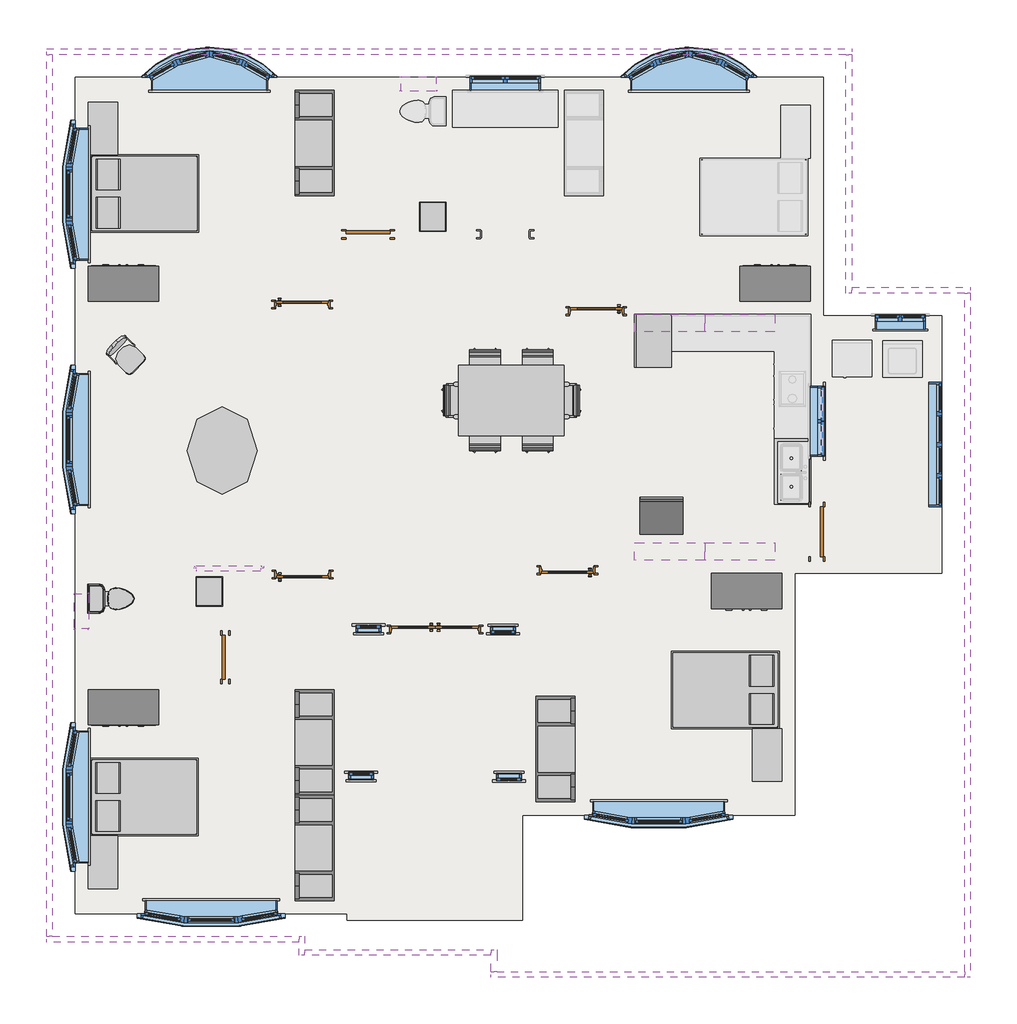
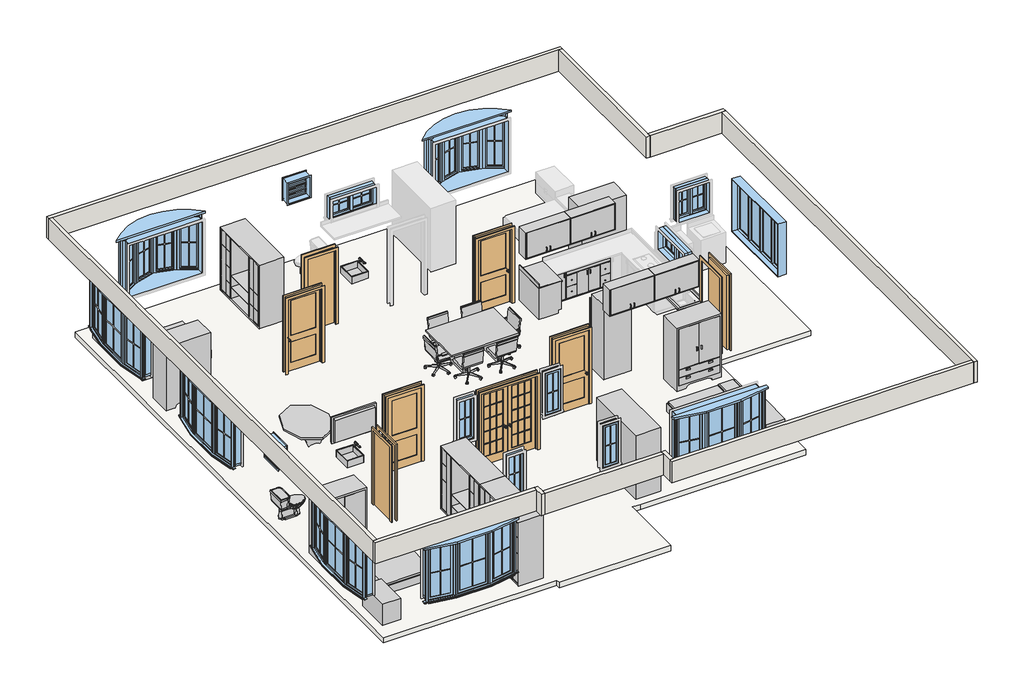
# One storey, part 1 of 2: 32 furniture elements, 17 windows, 10 walls, 8 doors, 3 flow terminals, 1 proxy, 1 slab.
"""IFC4 building model written with IfcOpenShell, lengths in millimetres."""

from ifc_helpers import new_model, si_unit, frame, origin, place, context, project, spatial, polyline, outline, extrude, faceted_brep, transform, mapped, element, save
from components import proxy_76352e5b, door_fac3bb52, door_d4071c8b, door_049a69ed, door_78caadf7, door_de72ddbf, flow_terminal_cce4e9d2, toilet_domestic_3d_toilet_domestic_3d_ba6479b0, toilet_domestic_3d_toilet_domestic_3d_30431060, furniture_b04c6994, furniture_ff3c2f57, furniture_b58f7881, furniture_6b884072, chair_task_chair_task_b7f3823b, chair_task_arms_chair_task_arms_fa5a08ef, furniture_4e2f607e, furniture_5f80dcf3, furniture_88072bd9, furniture_eb3a3c23, furniture_0bcc43ae, furniture_c105135d, furniture_5e39d705, furniture_ea954fa4, furniture_82e269c4, window_133af304, window_4630e4ac, window_bf21e6cb, window_ab94cc4f, window_791baf9d, window_a42194c0, window_f2d8fef0

model = new_model("IFC4")

# Units and contexts
model_context = context("Model", 3, world=origin())
ifc_project = project(units=[si_unit("LENGTHUNIT", "METRE", prefix="MILLI")], contexts=[model_context])

# Site, building, storey
site = spatial("IfcSite", under=ifc_project)
building = spatial("IfcBuilding", under=site)
storey = spatial("IfcBuildingStorey", under=building, Elevation=914.4)

# Proxy
placement = place(None, origin())
proxy_shape = proxy_76352e5b(model_context)
element("IfcBuildingElementProxy", 1, Name="Refrigerator-Built-in : 30\" x 24\" LH", ObjectType="Refrigerator-Built-in : 30\" x 24\" LH", at=placement, inside=storey, context=model_context, shape_type="MappedRepresentation", body=[
    mapped(proxy_shape, transform((-9990.4494093, 7653.8997772, 914.4), x_axis=(1.0, 0.0, 0.0), y_axis=(0.0, 1.0, 0.0), z_axis=(0.0, 0.0, 1.0))),
])

# Doors
door_shape = door_fac3bb52(model_context)
element("IfcDoor", 2, ObjectType="Door-Interior-Double-Full Glass-Wood : 60\" x 84\"", at=placement, inside=storey, context=model_context, shape_type="MappedRepresentation", body=[
    mapped(door_shape, transform((-13921.0994093, 5718.3487487, 914.4), x_axis=(1.0, 0.0, 0.0), y_axis=(0.0, 1.0, 0.0), z_axis=(0.0, 0.0, 1.0))),
])
door_2_shape = door_d4071c8b(model_context)
element("IfcDoor", 3, ObjectType="Door-Interior-Single-2_Panel-Wood : 36\" x 84\"", at=placement, inside=storey, context=model_context, shape_type="MappedRepresentation", body=[
    mapped(door_2_shape, transform((-16226.1494093, 11357.1487487, 914.4), x_axis=(1.0, 0.0, 0.0), y_axis=(0.0, 1.0, 0.0), z_axis=(0.0, 0.0, 1.0))),
])
element("IfcDoor", 4, ObjectType="Door-Interior-Single-2_Panel-Wood : 36\" x 84\"", at=placement, inside=storey, context=model_context, shape_type="MappedRepresentation", body=[
    mapped(door_2_shape, transform((-11622.3994093, 6740.6987487, 914.4), x_axis=(-1.0, 0.0, 0.0), y_axis=(0.0, -1.0, 0.0), z_axis=(0.0, 0.0, 1.0))),
])
door_3_shape = door_049a69ed(model_context)
element("IfcDoor", 5, ObjectType="Door-Interior-Single-2_Panel-Wood : 36\" x 84\"", at=placement, inside=storey, context=model_context, shape_type="MappedRepresentation", body=[
    mapped(door_3_shape, transform((-11120.7494093, 11242.8487487, 914.4), x_axis=(-1.0, 0.0, 0.0), y_axis=(0.0, -1.0, 0.0), z_axis=(0.0, 0.0, 1.0))),
])
element("IfcDoor", 6, ObjectType="Door-Interior-Single-2_Panel-Wood : 36\" x 84\"", at=placement, inside=storey, context=model_context, shape_type="MappedRepresentation", body=[
    mapped(door_3_shape, transform((-16219.7994093, 6664.4987487, 914.4), x_axis=(1.0, 0.0, 0.0), y_axis=(0.0, 1.0, 0.0), z_axis=(0.0, 0.0, 1.0))),
])
door_4_shape = door_78caadf7(model_context)
element("IfcDoor", 7, ObjectType="Single-Flush : 30\" x 84\"", at=placement, inside=storey, context=model_context, shape_type="MappedRepresentation", body=[
    mapped(door_4_shape, transform((-15083.1494093, 12573.1737487, 914.4), x_axis=(-1.0, 0.0, 0.0), y_axis=(0.0, -1.0, 0.0), z_axis=(0.0, 0.0, 1.0))),
])
element("IfcDoor", 8, ObjectType="Single-Flush : 30\" x 84\"", at=placement, inside=storey, context=model_context, shape_type="MappedRepresentation", body=[
    mapped(door_4_shape, transform((-17559.6494093, 5232.5737487, 914.4), x_axis=(0.0, -1.0, 0.0), y_axis=(1.0, 0.0, 0.0), z_axis=(0.0, 0.0, 1.0))),
])
door_5_shape = door_de72ddbf(model_context)
element("IfcDoor", 9, ObjectType="Single-Flush : 34\" x 84\"", at=placement, inside=storey, context=model_context, shape_type="MappedRepresentation", body=[
    mapped(door_5_shape, transform((-7291.6994093, 7410.6237487, 914.4), x_axis=(0.0, -1.0, 0.0), y_axis=(1.0, 0.0, 0.0), z_axis=(0.0, 0.0, 1.0))),
])

# Flow terminals
flow_terminal_shape = flow_terminal_cce4e9d2(model_context)
element("IfcFlowTerminal", 10, ObjectType="Sink - Work : 20\"x18\"", at=placement, inside=storey, context=model_context, shape_type="MappedRepresentation", body=[
    mapped(flow_terminal_shape, transform((-13730.5994093, 12877.9737487, 1828.8), x_axis=(0.0, -1.0, 0.0), y_axis=(1.0, 0.0, 0.0), z_axis=(0.0, 0.0, 1.0))),
])
element("IfcFlowTerminal", 11, ObjectType="Sink - Work : 20\"x18\"", at=placement, inside=storey, context=model_context, shape_type="MappedRepresentation", body=[
    mapped(flow_terminal_shape, transform((-17610.4494093, 6375.5737487, 1828.8), x_axis=(0.0, -1.0, 0.0), y_axis=(1.0, 0.0, 0.0), z_axis=(0.0, 0.0, 1.0))),
])
toilet_domestic_3d_toilet_domestic_3d_shape = toilet_domestic_3d_toilet_domestic_3d_ba6479b0(model_context)
toilet_domestic_3d_toilet_domestic_3d_2_shape = toilet_domestic_3d_toilet_domestic_3d_30431060(model_context)
element("IfcFlowTerminal", 12, ObjectType="Toilet-Domestic-3D : Toilet-Domestic-3D", at=placement, inside=storey, context=model_context, shape_type="MappedRepresentation", body=[
    mapped(toilet_domestic_3d_toilet_domestic_3d_shape, transform((-19451.3454366, 6248.5737487, 914.4), x_axis=(0.0, 1.0, 0.0), y_axis=(-1.0, 0.0, 0.0), z_axis=(0.0, 0.0, 1.0))),
    mapped(toilet_domestic_3d_toilet_domestic_3d_2_shape, transform((-19451.3454366, 6248.5737487, 914.4), x_axis=(0.0, 1.0, 0.0), y_axis=(-1.0, 0.0, 0.0), z_axis=(0.0, 0.0, 1.0))),
])

# Furniture
furniture_shape = furniture_b04c6994(model_context)
element("IfcFurniture", 13, ObjectType="48\" 2", at=placement, inside=storey, context=model_context, shape_type="MappedRepresentation", body=[
    mapped(furniture_shape, transform((-9020.8443693, 11182.5237487, 914.4), x_axis=(1.0, 0.0, 0.0), y_axis=(0.0, 1.0, 0.0), z_axis=(0.0, 0.0, 1.0))),
])
furniture_2_shape = furniture_ff3c2f57(model_context)
element("IfcFurniture", 14, ObjectType="Base Cabinet-Corner Unit-Square : 36\" 2", at=placement, inside=storey, context=model_context, shape_type="MappedRepresentation", body=[
    mapped(furniture_2_shape, transform((-10453.9994093, 10655.7860438, 914.4), x_axis=(0.0, 1.0, 0.0), y_axis=(-1.0, 0.0, 0.0), z_axis=(0.0, 0.0, 1.0))),
])
furniture_3_shape = furniture_b58f7881(model_context)
element("IfcFurniture", 15, ObjectType="Bed-Box : Double 53\" x 74\"", at=placement, inside=storey, context=model_context, shape_type="MappedRepresentation", body=[
    mapped(furniture_3_shape, transform((-19197.4289175, 12938.8712897, 914.4), x_axis=(0.0, 1.0, 0.0), y_axis=(-1.0, 0.0, 0.0), z_axis=(0.0, 0.0, 1.0))),
])
element("IfcFurniture", 16, ObjectType="Bed-Box : Double 53\" x 74\"", at=placement, inside=storey, context=model_context, shape_type="MappedRepresentation", body=[
    mapped(furniture_3_shape, transform((-19203.7789175, 2467.7212897, 914.4), x_axis=(0.0, 1.0, 0.0), y_axis=(-1.0, 0.0, 0.0), z_axis=(0.0, 0.0, 1.0))),
])
element("IfcFurniture", 17, ObjectType="Bed-Box : Double 53\" x 74\"", at=placement, inside=storey, context=model_context, shape_type="MappedRepresentation", body=[
    mapped(furniture_3_shape, transform((-8644.7699011, 5006.5762077, 914.4), x_axis=(0.0, -1.0, 0.0), y_axis=(1.0, 0.0, 0.0), z_axis=(0.0, 0.0, 1.0))),
])
furniture_4_shape = furniture_6b884072(model_context)
element("IfcFurniture", 18, ObjectType="Cabinet File-Lateral 2 Drawer : 36\" x 20\" x 24\"", at=placement, inside=storey, context=model_context, shape_type="MappedRepresentation", body=[
    mapped(furniture_4_shape, transform((-20621.2177854, 14588.3462626, 914.4), x_axis=(0.0, 1.0, 0.0), y_axis=(-1.0, 0.0, 0.0), z_axis=(0.0, 0.0, 1.0))),
])
element("IfcFurniture", 19, ObjectType="Cabinet File-Lateral 2 Drawer : 36\" x 20\" x 24\"", at=placement, inside=storey, context=model_context, shape_type="MappedRepresentation", body=[
    mapped(furniture_4_shape, transform((-20621.2177854, 1856.5962626, 914.4), x_axis=(0.0, 1.0, 0.0), y_axis=(-1.0, 0.0, 0.0), z_axis=(0.0, 0.0, 1.0))),
])
element("IfcFurniture", 20, ObjectType="Cabinet File-Lateral 2 Drawer : 36\" x 20\" x 24\"", at=placement, inside=storey, context=model_context, shape_type="MappedRepresentation", body=[
    mapped(furniture_4_shape, transform((-7220.9810332, 3357.1012348, 914.4), x_axis=(0.0, -1.0, 0.0), y_axis=(1.0, 0.0, 0.0), z_axis=(0.0, 0.0, 1.0))),
])
chair_task_chair_task_shape = chair_task_chair_task_b7f3823b(model_context)
element("IfcFurniture", 21, ObjectType="Chair-Task : Chair-Task", at=placement, inside=storey, context=model_context, shape_type="MappedRepresentation", body=[
    mapped(chair_task_chair_task_shape, transform((-11995.7585896, 10318.8196503, 914.4), x_axis=(-1.0, 0.0, 0.0), y_axis=(0.0, -1.0, 0.0), z_axis=(0.0, 0.0, 1.0))),
])
element("IfcFurniture", 22, ObjectType="Chair-Task : Chair-Task", at=placement, inside=storey, context=model_context, shape_type="MappedRepresentation", body=[
    mapped(chair_task_chair_task_shape, transform((-12277.740229, 9061.7278471, 914.4), x_axis=(1.0, 0.0, 0.0), y_axis=(0.0, 1.0, 0.0), z_axis=(0.0, 0.0, 1.0))),
])
element("IfcFurniture", 23, ObjectType="Chair-Task : Chair-Task", at=placement, inside=storey, context=model_context, shape_type="MappedRepresentation", body=[
    mapped(chair_task_chair_task_shape, transform((-12910.1585896, 10318.8196503, 914.4), x_axis=(-1.0, 0.0, 0.0), y_axis=(0.0, -1.0, 0.0), z_axis=(0.0, 0.0, 1.0))),
])
element("IfcFurniture", 24, ObjectType="Chair-Task : Chair-Task", at=placement, inside=storey, context=model_context, shape_type="MappedRepresentation", body=[
    mapped(chair_task_chair_task_shape, transform((-13192.140229, 9061.7278471, 914.4), x_axis=(1.0, 0.0, 0.0), y_axis=(0.0, 1.0, 0.0), z_axis=(0.0, 0.0, 1.0))),
])
chair_task_arms_chair_task_arms_shape = chair_task_arms_chair_task_arms_fa5a08ef(model_context)
element("IfcFurniture", 25, ObjectType="Chair-Task Arms : Chair-Task Arms", at=placement, inside=storey, context=model_context, shape_type="MappedRepresentation", body=[
    mapped(chair_task_arms_chair_task_arms_shape, transform((-13527.2953109, 9831.2645684, 914.4), x_axis=(0.0, -1.0, 0.0), y_axis=(1.0, 0.0, 0.0), z_axis=(0.0, 0.0, 1.0))),
])
element("IfcFurniture", 26, ObjectType="Chair-Task Arms : Chair-Task Arms", at=placement, inside=storey, context=model_context, shape_type="MappedRepresentation", body=[
    mapped(chair_task_arms_chair_task_arms_shape, transform((-11660.6035077, 9549.282929, 914.4), x_axis=(0.0, 1.0, 0.0), y_axis=(-1.0, 0.0, 0.0), z_axis=(0.0, 0.0, 1.0))),
])
furniture_5_shape = furniture_4e2f607e(model_context)
element("IfcFurniture", 27, ObjectType="Counter Top : 24\" Depth", at=placement, inside=storey, context=model_context, shape_type="MappedRepresentation", body=[
    mapped(furniture_5_shape, transform((-10453.9994093, 11468.5860438, 914.4), x_axis=(0.0, 1.0, 0.0), y_axis=(-1.0, 0.0, 0.0), z_axis=(0.0, 0.0, 1.0))),
])
furniture_6_shape = furniture_5f80dcf3(model_context)
element("IfcFurniture", 28, ObjectType="Counter Top w Sink : 24\" Depth", at=placement, inside=storey, context=model_context, shape_type="MappedRepresentation", body=[
    mapped(furniture_6_shape, transform((-7393.2994093, 7823.0614536, 914.4), x_axis=(0.0, -1.0, 0.0), y_axis=(1.0, 0.0, 0.0), z_axis=(0.0, 0.0, 1.0))),
])
furniture_7_shape = furniture_88072bd9(model_context)
element("IfcFurniture", 29, ObjectType="Entertainment Center.0001 : 72\" x 72\" x 24\"", at=placement, inside=storey, context=model_context, shape_type="MappedRepresentation", body=[
    mapped(furniture_7_shape, transform((-15572.0994093, 14154.3237487, 914.4), x_axis=(0.0, -1.0, 0.0), y_axis=(1.0, 0.0, 0.0), z_axis=(0.0, 0.0, 1.0))),
])
element("IfcFurniture", 30, ObjectType="Entertainment Center.0001 : 72\" x 72\" x 24\"", at=placement, inside=storey, context=model_context, shape_type="MappedRepresentation", body=[
    mapped(furniture_7_shape, transform((-12270.0994093, 3638.7237487, 914.4), x_axis=(0.0, 1.0, 0.0), y_axis=(-1.0, 0.0, 0.0), z_axis=(0.0, 0.0, 1.0))),
])
element("IfcFurniture", 31, ObjectType="Entertainment Center.0001 : 72\" x 72\" x 24\"", at=placement, inside=storey, context=model_context, shape_type="MappedRepresentation", body=[
    mapped(furniture_7_shape, transform((-15572.0994093, 1924.2237487, 914.4), x_axis=(0.0, -1.0, 0.0), y_axis=(1.0, 0.0, 0.0), z_axis=(0.0, 0.0, 1.0))),
])
element("IfcFurniture", 32, ObjectType="Entertainment Center.0001 : 72\" x 72\" x 24\"", at=placement, inside=storey, context=model_context, shape_type="MappedRepresentation", body=[
    mapped(furniture_7_shape, transform((-15572.0994093, 3753.0237487, 914.4), x_axis=(0.0, -1.0, 0.0), y_axis=(1.0, 0.0, 0.0), z_axis=(0.0, 0.0, 1.0))),
])
furniture_8_shape = furniture_eb3a3c23(model_context)
element("IfcFurniture", 33, ObjectType="Seating-Auditorium : 18\" x 24\" x 30\"", at=placement, inside=storey, context=model_context, shape_type="MappedRepresentation", body=[
    mapped(furniture_8_shape, transform((-19310.9207256, 10729.9667219, 914.4), x_axis=(-0.7071067811865499, -0.7071067811865454, 0.0), y_axis=(0.7071067811865454, -0.7071067811865499, 0.0), z_axis=(0.0, 0.0, 1.0))),
])
furniture_9_shape = furniture_0bcc43ae(model_context)
element("IfcFurniture", 34, ObjectType="Table-Conference2 w Chairs : 48\" x 144\" 2", at=placement, inside=storey, context=model_context, shape_type="MappedRepresentation", body=[
    mapped(furniture_9_shape, transform((-12593.9494093, 9690.2737487, 914.4), x_axis=(1.0, 0.0, 0.0), y_axis=(0.0, 1.0, 0.0), z_axis=(0.0, 0.0, 1.0))),
])
furniture_10_shape = furniture_c105135d(model_context)
element("IfcFurniture", 35, ObjectType="Table-Ellipse : 60\" x 48\" 2", at=placement, inside=storey, context=model_context, shape_type="MappedRepresentation", body=[
    mapped(furniture_10_shape, transform((-17616.7994093, 8820.3237487, 914.4), x_axis=(0.0, 1.0, 0.0), y_axis=(-1.0, 0.0, 0.0), z_axis=(0.0, 0.0, 1.0))),
])
furniture_11_shape = furniture_5e39d705(model_context)
element("IfcFurniture", 36, ObjectType="Television-Plasma : 50\" 2", at=placement, inside=storey, context=model_context, shape_type="MappedRepresentation", body=[
    mapped(furniture_11_shape, transform((-17445.3494093, 6724.8237487, 2133.6), x_axis=(-1.0, 0.0, 0.0), y_axis=(0.0, -1.0, 0.0), z_axis=(0.0, 0.0, 1.0))),
])
furniture_12_shape = furniture_ea954fa4(model_context)
element("IfcFurniture", 37, ObjectType="Upper Cabinet-Pass-Thru : 48\" x 30\" x 12\"", at=placement, inside=storey, context=model_context, shape_type="MappedRepresentation", body=[
    mapped(furniture_12_shape, transform((-9825.6617044, 6915.3237487, 1676.4), x_axis=(-1.0, 0.0, 0.0), y_axis=(0.0, -1.0, 0.0), z_axis=(0.0, 0.0, 1.0))),
])
element("IfcFurniture", 38, ObjectType="Upper Cabinet-Pass-Thru : 48\" x 30\" x 12\"", at=placement, inside=storey, context=model_context, shape_type="MappedRepresentation", body=[
    mapped(furniture_12_shape, transform((-8606.4617044, 6915.3237487, 1676.4), x_axis=(-1.0, 0.0, 0.0), y_axis=(0.0, -1.0, 0.0), z_axis=(0.0, 0.0, 1.0))),
])
element("IfcFurniture", 39, ObjectType="Upper Cabinet-Pass-Thru : 48\" x 30\" x 12\"", at=placement, inside=storey, context=model_context, shape_type="MappedRepresentation", body=[
    mapped(furniture_12_shape, transform((-9863.1371142, 11182.5237487, 914.4), x_axis=(1.0, 0.0, 0.0), y_axis=(0.0, 1.0, 0.0), z_axis=(0.0, 0.0, 1.0))),
])
element("IfcFurniture", 40, ObjectType="Upper Cabinet-Pass-Thru : 48\" x 30\" x 12\"", at=placement, inside=storey, context=model_context, shape_type="MappedRepresentation", body=[
    mapped(furniture_12_shape, transform((-8643.9371142, 11182.5237487, 914.4), x_axis=(1.0, 0.0, 0.0), y_axis=(0.0, 1.0, 0.0), z_axis=(0.0, 0.0, 1.0))),
])
furniture_13_shape = furniture_82e269c4(model_context)
element("IfcFurniture", 41, ObjectType="Wardrobe : 48\" x 72\" x 24\"", at=placement, inside=storey, context=model_context, shape_type="MappedRepresentation", body=[
    mapped(furniture_13_shape, transform((-8241.7061495, 6965.6625583, 914.4), x_axis=(1.0, 0.0, 0.0), y_axis=(0.0, 1.0, 0.0), z_axis=(0.0, 0.0, 1.0))),
])
element("IfcFurniture", 42, ObjectType="Wardrobe : 48\" x 72\" x 24\"", at=placement, inside=storey, context=model_context, shape_type="MappedRepresentation", body=[
    mapped(furniture_13_shape, transform((-19062.1061495, 4946.3625583, 914.4), x_axis=(1.0, 0.0, 0.0), y_axis=(0.0, 1.0, 0.0), z_axis=(0.0, 0.0, 1.0))),
])
element("IfcFurniture", 43, ObjectType="Wardrobe : 48\" x 72\" x 24\"", at=placement, inside=storey, context=model_context, shape_type="MappedRepresentation", body=[
    mapped(furniture_13_shape, transform((-19600.4926691, 11132.1849391, 914.4), x_axis=(-1.0, 0.0, 0.0), y_axis=(0.0, -1.0, 0.0), z_axis=(0.0, 0.0, 1.0))),
])
element("IfcFurniture", 44, ObjectType="Wardrobe : 48\" x 72\" x 24\"", at=placement, inside=storey, context=model_context, shape_type="MappedRepresentation", body=[
    mapped(furniture_13_shape, transform((-8284.7926691, 11132.1849391, 914.4), x_axis=(-1.0, 0.0, 0.0), y_axis=(0.0, -1.0, 0.0), z_axis=(0.0, 0.0, 1.0))),
])

# Slab
element("IfcSlab", 45, ObjectType="Generic - 6\"", at=placement, inside=storey, context=model_context, shape_type="SweptSolid", body=[
    extrude(outline(polyline([(-7177.3994093, 15297.3237487), (-7177.3994093, 11157.1237487), (-5119.9994093, 11157.1237487), (-5119.9994093, 6686.7237487), (-7672.6994093, 6686.7237487), (-7672.6994093, 2495.7237487), (-12168.4994093, 2495.7237487), (-12397.0994093, 2495.7237487), (-12397.0994093, 666.9237487), (-15445.0994093, 666.9237487), (-15445.0994093, 781.2237487), (-20169.4994093, 781.2237487), (-20169.4994093, 15297.3237487), (-7177.3994093, 15297.3237487)])), frame((0.0, 0.0, 762.0), z_axis=(0.0, 0.0, 1.0), x_axis=(1.0, 0.0, 0.0)), (0.0, 0.0, 1.0), 152.4),
])

# Walls
element("IfcWall", 46, at=placement, inside=storey, context=model_context, shape_type="Brep", body=[
    faceted_brep([(-20664.7994093, 15691.0237487, 3505.2), (-20563.1994093, 15691.0237487, 3505.2), (-6783.6994093, 15691.0237487, 3505.2), (-6682.0994093, 15691.0237487, 3505.2), (-6682.0994093, 15691.0237487, 4114.8), (-6783.6994093, 15691.0237487, 4114.8), (-20563.1994093, 15691.0237487, 4114.8), (-20664.7994093, 15691.0237487, 4114.8), (-20664.7994093, 15792.6237487, 3505.2), (-20664.7994093, 15792.6237487, 4114.8), (-6682.0994093, 15792.6237487, 4114.8), (-6682.0994093, 15792.6237487, 3505.2)], [[[0, 1, 2, 3, 4, 5, 6, 7]], [[8, 9, 10, 11]], [[3, 2, 1, 0, 8, 11]], [[7, 6, 5, 4, 10, 9]], [[4, 3, 11, 10]], [[0, 7, 9, 8]]]),
])
element("IfcWall", 47, at=placement, inside=storey, context=model_context, shape_type="Brep", body=[
    faceted_brep([(-6783.6994093, 15691.0237487, 3505.2), (-6783.6994093, 11550.8237487, 3505.2), (-6783.6994093, 11550.8237487, 4114.8), (-6783.6994093, 15691.0237487, 4114.8), (-6682.0994093, 15691.0237487, 3505.2), (-6682.0994093, 15691.0237487, 4114.8), (-6682.0994093, 11652.4237487, 4114.8), (-6682.0994093, 11550.8237487, 4114.8), (-6682.0994093, 11550.8237487, 3505.2), (-6682.0994093, 11652.4237487, 3505.2)], [[[0, 1, 2, 3]], [[4, 5, 6, 7, 8, 9]], [[1, 0, 4, 9, 8]], [[3, 2, 7, 6, 5]], [[0, 3, 5, 4]], [[2, 1, 8, 7]]]),
])
element("IfcWall", 48, at=placement, inside=storey, context=model_context, shape_type="Brep", body=[
    faceted_brep([(-6682.0994093, 11550.8237487, 3505.2), (-4726.2994093, 11550.8237487, 3505.2), (-4624.6994093, 11550.8237487, 3505.2), (-4624.6994093, 11550.8237487, 4114.8), (-4726.2994093, 11550.8237487, 4114.8), (-6682.0994093, 11550.8237487, 4114.8), (-6682.0994093, 11652.4237487, 3505.2), (-6682.0994093, 11652.4237487, 4114.8), (-4624.6994093, 11652.4237487, 4114.8), (-4624.6994093, 11652.4237487, 3505.2)], [[[0, 1, 2, 3, 4, 5]], [[6, 7, 8, 9]], [[2, 1, 0, 6, 9]], [[5, 4, 3, 8, 7]], [[0, 5, 7, 6]], [[3, 2, 9, 8]]]),
])
element("IfcWall", 49, at=placement, inside=storey, context=model_context, shape_type="Brep", body=[
    faceted_brep([(-4726.2994093, 11550.8237487, 3505.2), (-4726.2994093, -222.0762513, 3505.2), (-4726.2994093, -323.6762513, 3505.2), (-4726.2994093, -323.6762513, 4114.8), (-4726.2994093, -222.0762513, 4114.8), (-4726.2994093, 11550.8237487, 4114.8), (-4624.6994093, 11550.8237487, 3505.2), (-4624.6994093, 11550.8237487, 4114.8), (-4624.6994093, -323.6762513, 4114.8), (-4624.6994093, -323.6762513, 3505.2)], [[[0, 1, 2, 3, 4, 5]], [[6, 7, 8, 9]], [[2, 1, 0, 6, 9]], [[5, 4, 3, 8, 7]], [[0, 5, 7, 6]], [[3, 2, 9, 8]]]),
])
element("IfcWall", 50, at=placement, inside=storey, context=model_context, shape_type="Brep", body=[
    faceted_brep([(-4726.2994093, -222.0762513, 3505.2), (-12847.9494093, -222.0762513, 3505.2), (-12949.5494093, -222.0762513, 3505.2), (-12949.5494093, -222.0762513, 4114.8), (-12847.9494093, -222.0762513, 4114.8), (-4726.2994093, -222.0762513, 4114.8), (-4726.2994093, -323.6762513, 3505.2), (-4726.2994093, -323.6762513, 4114.8), (-12949.5494093, -323.6762513, 4114.8), (-12949.5494093, -323.6762513, 3505.2)], [[[0, 1, 2, 3, 4, 5]], [[6, 7, 8, 9]], [[2, 1, 0, 6, 9]], [[5, 4, 3, 8, 7]], [[0, 5, 7, 6]], [[3, 2, 9, 8]]]),
])
element("IfcWall", 51, at=placement, inside=storey, context=model_context, shape_type="Brep", body=[
    faceted_brep([(-12847.9494093, -222.0762513, 3505.2), (-12847.9494093, 158.9237487, 3505.2), (-12847.9494093, 158.9237487, 4114.8), (-12847.9494093, -222.0762513, 4114.8), (-12949.5494093, -222.0762513, 3505.2), (-12949.5494093, -222.0762513, 4114.8), (-12949.5494093, 57.3237487, 4114.8), (-12949.5494093, 158.9237487, 4114.8), (-12949.5494093, 158.9237487, 3505.2), (-12949.5494093, 57.3237487, 3505.2)], [[[0, 1, 2, 3]], [[4, 5, 6, 7, 8, 9]], [[1, 0, 4, 9, 8]], [[3, 2, 7, 6, 5]], [[0, 3, 5, 4]], [[2, 1, 8, 7]]]),
])
element("IfcWall", 52, at=placement, inside=storey, context=model_context, shape_type="SweptSolid", body=[
    extrude(outline(polyline([(-16181.6994093, 158.9237487), (-12949.5494093, 158.9237487), (-12949.5494093, 57.3237487), (-16181.6994093, 57.3237487), (-16181.6994093, 158.9237487)])), frame((0.0, 0.0, 3505.2), z_axis=(0.0, 0.0, 1.0), x_axis=(1.0, 0.0, 0.0)), (0.0, 0.0, 1.0), 609.6),
])
element("IfcWall", 53, at=placement, inside=storey, context=model_context, shape_type="Brep", body=[
    faceted_brep([(-16181.6994093, 57.3237487, 3505.2), (-16181.6994093, 158.9237487, 3505.2), (-16181.6994093, 387.5237487, 3505.2), (-16181.6994093, 387.5237487, 4114.8), (-16181.6994093, 158.9237487, 4114.8), (-16181.6994093, 57.3237487, 4114.8), (-16283.2994093, 57.3237487, 3505.2), (-16283.2994093, 57.3237487, 4114.8), (-16283.2994093, 285.9237487, 4114.8), (-16283.2994093, 387.5237487, 4114.8), (-16283.2994093, 387.5237487, 3505.2), (-16283.2994093, 285.9237487, 3505.2)], [[[0, 1, 2, 3, 4, 5]], [[6, 7, 8, 9, 10, 11]], [[2, 1, 0, 6, 11, 10]], [[5, 4, 3, 9, 8, 7]], [[0, 5, 7, 6]], [[3, 2, 10, 9]]]),
])
element("IfcWall", 54, at=placement, inside=storey, context=model_context, shape_type="Brep", body=[
    faceted_brep([(-16283.2994093, 387.5237487, 3505.2), (-20563.1994093, 387.5237487, 3505.2), (-20664.7994093, 387.5237487, 3505.2), (-20664.7994093, 387.5237487, 4114.8), (-20563.1994093, 387.5237487, 4114.8), (-16283.2994093, 387.5237487, 4114.8), (-16283.2994093, 285.9237487, 3505.2), (-16283.2994093, 285.9237487, 4114.8), (-20664.7994093, 285.9237487, 4114.8), (-20664.7994093, 285.9237487, 3505.2)], [[[0, 1, 2, 3, 4, 5]], [[6, 7, 8, 9]], [[2, 1, 0, 6, 9]], [[5, 4, 3, 8, 7]], [[0, 5, 7, 6]], [[3, 2, 9, 8]]]),
])
element("IfcWall", 55, at=placement, inside=storey, context=model_context, shape_type="SweptSolid", body=[
    extrude(outline(polyline([(-20563.1994093, 15691.0237487), (-20563.1994093, 387.5237487), (-20664.7994093, 387.5237487), (-20664.7994093, 15691.0237487), (-20563.1994093, 15691.0237487)])), frame((0.0, 0.0, 3505.2), z_axis=(0.0, 0.0, 1.0), x_axis=(1.0, 0.0, 0.0)), (0.0, 0.0, 1.0), 609.6),
])

# Windows
window_shape = window_133af304(model_context)
element("IfcWindow", 56, ObjectType="Window-Awning-Double-Horizontal : 48\" x 24\"", at=placement, inside=storey, context=model_context, shape_type="MappedRepresentation", body=[
    mapped(window_shape, transform((-12701.8994093, 15183.0237487, 914.4), x_axis=(1.0, 0.0, 0.0), y_axis=(0.0, 1.0, 0.0), z_axis=(0.0, 0.0, 1.0))),
])
element("IfcWindow", 57, ObjectType="Window-Awning-Double-Horizontal : 48\" x 24\"", at=placement, inside=storey, context=model_context, shape_type="MappedRepresentation", body=[
    mapped(window_shape, transform((-7291.6994093, 9328.3237487, 1155.7), x_axis=(0.0, -1.0, 0.0), y_axis=(1.0, 0.0, 0.0), z_axis=(0.0, 0.0, 1.0))),
])
window_2_shape = window_4630e4ac(model_context)
element("IfcWindow", 58, ObjectType="Window-Awning-Single : 17\" x 48\"", at=placement, inside=storey, context=model_context, shape_type="MappedRepresentation", body=[
    mapped(window_2_shape, transform((-12638.3994093, 3162.4737487, 914.4), x_axis=(-1.0, 0.0, 0.0), y_axis=(0.0, -1.0, 0.0), z_axis=(0.0, 0.0, 1.0))),
])
element("IfcWindow", 59, ObjectType="Window-Awning-Single : 17\" x 48\"", at=placement, inside=storey, context=model_context, shape_type="MappedRepresentation", body=[
    mapped(window_2_shape, transform((-15203.7994093, 3162.4737487, 914.4), x_axis=(1.0, 0.0, 0.0), y_axis=(0.0, 1.0, 0.0), z_axis=(0.0, 0.0, 1.0))),
])
element("IfcWindow", 60, ObjectType="Window-Awning-Single : 17\" x 48\"", at=placement, inside=storey, context=model_context, shape_type="MappedRepresentation", body=[
    mapped(window_2_shape, transform((-15076.7994093, 5715.1737487, 914.4), x_axis=(1.0, 0.0, 0.0), y_axis=(0.0, 1.0, 0.0), z_axis=(0.0, 0.0, 1.0))),
])
element("IfcWindow", 61, ObjectType="Window-Awning-Single : 17\" x 48\"", at=placement, inside=storey, context=model_context, shape_type="MappedRepresentation", body=[
    mapped(window_2_shape, transform((-12739.9994093, 5715.1737487, 914.4), x_axis=(-1.0, 0.0, 0.0), y_axis=(0.0, -1.0, 0.0), z_axis=(0.0, 0.0, 1.0))),
])
window_3_shape = window_bf21e6cb(model_context)
element("IfcWindow", 62, ObjectType="Window-Bay-Casement-10_Degree_Angle : 90\" x 60\" x 6\"", at=placement, inside=storey, context=model_context, shape_type="MappedRepresentation", body=[
    mapped(window_3_shape, transform((-20055.1994093, 13268.4987487, 914.4), x_axis=(0.0, 1.0, 0.0), y_axis=(-1.0, 0.0, 0.0), z_axis=(0.0, 0.0, 1.0))),
])
element("IfcWindow", 63, ObjectType="Window-Bay-Casement-10_Degree_Angle : 90\" x 60\" x 6\"", at=placement, inside=storey, context=model_context, shape_type="MappedRepresentation", body=[
    mapped(window_3_shape, transform((-20055.1994093, 9010.8237487, 914.4), x_axis=(0.0, 1.0, 0.0), y_axis=(-1.0, 0.0, 0.0), z_axis=(0.0, 0.0, 1.0))),
])
element("IfcWindow", 64, ObjectType="Window-Bay-Casement-10_Degree_Angle : 90\" x 60\" x 6\"", at=placement, inside=storey, context=model_context, shape_type="MappedRepresentation", body=[
    mapped(window_3_shape, transform((-20055.1994093, 2810.0487487, 914.4), x_axis=(0.0, 1.0, 0.0), y_axis=(-1.0, 0.0, 0.0), z_axis=(0.0, 0.0, 1.0))),
])
element("IfcWindow", 65, ObjectType="Window-Bay-Casement-10_Degree_Angle : 90\" x 60\" x 6\"", at=placement, inside=storey, context=model_context, shape_type="MappedRepresentation", body=[
    mapped(window_3_shape, transform((-17807.2994093, 895.5237487, 914.4), x_axis=(-1.0, 0.0, 0.0), y_axis=(0.0, -1.0, 0.0), z_axis=(0.0, 0.0, 1.0))),
])
element("IfcWindow", 66, ObjectType="Window-Bay-Casement-10_Degree_Angle : 90\" x 60\" x 6\"", at=placement, inside=storey, context=model_context, shape_type="MappedRepresentation", body=[
    mapped(window_3_shape, transform((-10034.8994093, 2610.0237487, 914.4), x_axis=(-1.0, 0.0, 0.0), y_axis=(0.0, -1.0, 0.0), z_axis=(0.0, 0.0, 1.0))),
])
window_4_shape = window_ab94cc4f(model_context)
element("IfcWindow", 67, ObjectType="Window-Bow-Casement-15_Degree_Angle : 80\" x 60\"", at=placement, inside=storey, context=model_context, shape_type="MappedRepresentation", body=[
    mapped(window_4_shape, transform((-17835.8744093, 15183.0237487, 914.4), x_axis=(1.0, 0.0, 0.0), y_axis=(0.0, 1.0, 0.0), z_axis=(0.0, 0.0, 1.0))),
])
element("IfcWindow", 68, ObjectType="Window-Bow-Casement-15_Degree_Angle : 80\" x 60\"", at=placement, inside=storey, context=model_context, shape_type="MappedRepresentation", body=[
    mapped(window_4_shape, transform((-9511.0244093, 15183.0237487, 914.4), x_axis=(1.0, 0.0, 0.0), y_axis=(0.0, 1.0, 0.0), z_axis=(0.0, 0.0, 1.0))),
])
window_5_shape = window_791baf9d(model_context)
element("IfcWindow", 69, ObjectType="Window-Casement-Double : 34\" x 36\"", at=placement, inside=storey, context=model_context, shape_type="MappedRepresentation", body=[
    mapped(window_5_shape, transform((-5843.8994093, 11042.8237487, 914.4), x_axis=(-1.0, 0.0, 0.0), y_axis=(0.0, -1.0, 0.0), z_axis=(0.0, 0.0, 1.0))),
])
window_6_shape = window_a42194c0(model_context)
element("IfcWindow", 70, ObjectType="Window-Casement-Multi-Sash-Horizontal : 85\" x 60\"", at=placement, inside=storey, context=model_context, shape_type="MappedRepresentation", body=[
    mapped(window_6_shape, transform((-5234.2994093, 8921.9237487, 914.4), x_axis=(0.0, -1.0, 0.0), y_axis=(1.0, 0.0, 0.0), z_axis=(0.0, 0.0, 1.0))),
])
window_7_shape = window_f2d8fef0(model_context)
element("IfcWindow", 71, ObjectType="Window-Louvers : 24\" x 24\"", at=placement, inside=storey, context=model_context, shape_type="MappedRepresentation", body=[
    mapped(window_7_shape, transform((-20061.5494093, 6032.6737487, 1828.8), x_axis=(0.0, 1.0, 0.0), y_axis=(-1.0, 0.0, 0.0), z_axis=(0.0, 0.0, 1.0))),
])
element("IfcWindow", 72, ObjectType="Window-Louvers : 24\" x 24\"", at=placement, inside=storey, context=model_context, shape_type="MappedRepresentation", body=[
    mapped(window_7_shape, transform((-14206.8494093, 15189.3737487, 1828.8), x_axis=(1.0, 0.0, 0.0), y_axis=(0.0, 1.0, 0.0), z_axis=(0.0, 0.0, 1.0))),
])

save(model, "model.ifc")

# Revit data of these elements
# Type "Refrigerator-Built-in : 30\" x 24\" LH"
#   Assembly Code = "E1090400"
#   Depth = 2' - 0"
#   Handle = 0' - 0 1/4"
#   Height = 7' - 0"
#   Top Door Height = 5' - 0"
#   Width = 2' - 5 1/2"
#   Material = Metal - Paint Finish - Ivory,Glossy
#   Default Elevation = 0
# Type "Door-Interior-Double-Full Glass-Wood : 60\" x 84\""
#   Type Mark = "9"
#   Assembly Code = "C1020300"
#   Analytic Construction = "French door, wood frame with single glass"
#   Top Rail = 0' - 4 11/16"
#   Thickness = 0' - 1 3/8"
#   Thermal Resistance (R) = 1.0696 (h·ft²·°F)/BTU
#   Swing Angle [instance default] = 90.00°
#   Stiles = 0' - 4 3/4"
#   Rough Width = 5' - 2"
#   Rough Height = 7' - 1"
#   Panel Width = 2' - 6"
#   Height = 7' - 0"
#   Width = 5' - 0"
#   Heat Transfer Coefficient (U) = 0.9350 BTU/(h·ft²·°F)
#   Bottom Rail = 0' - 9 1/8"
#   Show Grill [instance default] = yes
#   Trim Material = Cherry
#   Panel Material = Cherry
#   Frame Material = Cherry
#   Door Handle Material = Aluminum
#   Visual Light Transmittance = 0
#   Solar Heat Gain Coefficient = 0
#   Wall Closure = (empty or 0)
#   Function = (empty or 0)
# Type "Door-Interior-Single-2_Panel-Wood : 36\" x 84\""
#   Type Mark = "12"
#   Assembly Code = "C1020300"
#   Analytic Construction = "Wooden"
#   Top Rail = 0' - 4 11/16"
#   Thickness = 0' - 1 3/8"
#   Thermal Resistance (R) = 2.5876 (h·ft²·°F)/BTU
#   Swing Angle [instance default] = 90.00°
#   Stiles = 0' - 4 3/4"
#   Rough Width = 3' - 2"
#   Rough Height = 7' - 1"
#   Lock Rail = 0' - 7 1/2"
#   Height = 7' - 0"
#   Width = 3' - 0"
#   Heat Transfer Coefficient (U) = 0.3865 BTU/(h·ft²·°F)
#   Bottom Rail = 0' - 9 1/8"
#   Trim Material = Cherry
#   Panel Material = Cherry
#   Frame Material = Cherry
#   Door Handle Material = Aluminum
#   Visual Light Transmittance = 0
#   Solar Heat Gain Coefficient = 0
#   Wall Closure = (empty or 0)
#   Function = (empty or 0)
# Type "Single-Flush : 30\" x 84\""
#   Type Mark = "4"
#   Construction Type Id = "MDOOR"
#   Assembly Code = "C1020"
#   Analytic Construction = "Metal"
#   Thickness = 0' - 2"
#   Heat Transfer Coefficient (U) = 0.651978 BTU/(h·ft²·°F)
#   Height = 7' - 0"
#   Trim Projection Ext = 0' - 1"
#   Trim Projection Int = 0' - 1"
#   Trim Width = 0' - 3"
#   Width = 2' - 6"
#   Define Thermal Properties by = 1
#   Define Thermal Properties by = 1
#   Door Material = Door - Panel
#   Frame Material = Door - Frame
#   Visual Light Transmittance = 0
#   Solar Heat Gain Coefficient = 0
#   Function = (empty or 0)
#   Wall Closure = (empty or 0)
# Type "Single-Flush : 34\" x 84\""
#   Type Mark = "2"
#   Construction Type Id = "MDOOR"
#   Assembly Code = "C1020"
#   Analytic Construction = "Metal"
#   Thickness = 0' - 2"
#   Heat Transfer Coefficient (U) = 0.651978 BTU/(h·ft²·°F)
#   Height = 7' - 0"
#   Trim Projection Ext = 0' - 1"
#   Trim Projection Int = 0' - 1"
#   Trim Width = 0' - 3"
#   Width = 2' - 10"
#   Define Thermal Properties by = 1
#   Define Thermal Properties by = 1
#   Door Material = Door - Panel
#   Frame Material = Door - Frame
#   Visual Light Transmittance = 0
#   Solar Heat Gain Coefficient = 0
#   Function = (empty or 0)
#   Wall Closure = (empty or 0)
# Type "Sink - Work : 20\"x18\""
#   WFU = 2
#   Sink Width = 1' - 6"
#   Sink Length = 1' - 8"
#   Sink Depth = 0' - 8"
#   Sanitary Radius = 3/4"
#   Sanitary Diameter = 1 1/2"
#   Hot Water Radius = 1/4"
#   Hot Water Diameter = 1/2"
#   HWFU = 2.25
#   Flow Pressure [instance default] = 8.00 psi
#   Faucet Height = 1' - 1 5/8"
#   Cold Water Radius = 1/4"
#   Cold Water Diameter = 1/2"
#   CWFU = 2.25
#   Sink Material = none
#   Faucet Material = none
#   Default Elevation = 0
# Type "Toilet-Domestic-3D : Toilet-Domestic-3D"
#   Assembly Code = "D2010110"
#   Toilet - Bowl/Basin Material = Porcelain, Linen
#   Toilet - Seat Material = Laminate, Linen, Matte
#   Default Elevation = 0
# Type "48\" 2"
#   Assembly Code = "C1030410"
#   Depth = 2' - 0"
#   Height = 2' - 11 1/2"
#   Toe Depth = 0' - 3"
#   Toe Height = 0' - 3 1/2"
#   Width = 4' - 0"
#   Cabinet Material = none
#   Door/Drawer Material = none
#   Handle Material = Cabinets - Handles
#   Default Elevation = 0
# Type "Base Cabinet-Corner Unit-Square : 36\" 2"
#   Assembly Code = "C1030410"
#   Depth = 2' - 0"
#   Height = 2' - 11 1/2"
#   Toe Depth = 0' - 3"
#   Toe Height = 0' - 3 1/2"
#   Width = 3' - 0"
#   Cabinet Material = Cabinets
#   Door/Drawer Material = Cabinets
#   Handle Material = Cabinets - Handles
#   Default Elevation = 0
# Type "Bed-Box : Double 53\" x 74\""
#   Assembly Code = "E2020200"
#   Length = 6' - 2"
#   Width = 4' - 5"
#   Frame Material = Birch
#   Mattress Material = Linen, White
#   Default Elevation = 0
# Type "Cabinet File-Lateral 2 Drawer : 36\" x 20\" x 24\""
#   Assembly Code = "E2020200"
#   Depth = 1' - 8"
#   Height = 2' - 0"
#   Width = 3' - 0"
#   Material = Metal - Steel
#   Default Elevation = 0
# Type "Chair-Task : Chair-Task"
#   Assembly Code = "E2020200"
#   Base Material = Plastic - Black
#   Caster Material = Plastic - Black
#   Seat/Back Material = Textile - Slate Blue
#   Default Elevation = 0
# Type "Chair-Task Arms : Chair-Task Arms"
#   Assembly Code = "E2020200"
#   Base Material = Plastic - Black
#   Caster Material = Plastic - Black
#   Seat/Back Material = Textile - Slate Blue
#   Default Elevation = 0
# Type "Counter Top : 24\" Depth"
#   Assembly Code = "C1030400"
#   Counter Thickness = 0' - 1 1/2"
#   Depth = 2' - 1"
#   Height = 3' - 0"
#   Length [instance default] = 8' - 0"
#   Counter Top Material = none
#   Default Elevation = 0
# Type "Counter Top w Sink : 24\" Depth"
#   Assembly Code = "C1030400"
#   Counter Thickness = 0' - 1 1/2"
#   Depth = 2' - 1"
#   Height = 3' - 0"
#   Length [instance default] = 8' - 0"
#   Sink Location [instance default] = 2' - 0"
#   Sink Location To Wall [instance default] = 0' - 6"
#   Sink Opening Depth [instance default] = 1' - 3"
#   Sink Opening Width [instance default] = 3' - 3"
#   Counter Top Material = none
#   Default Elevation = 0
# Type "Entertainment Center.0001 : 72\" x 72\" x 24\""
#   Assembly Code = "E2020200"
#   Center Width = 2' - 8"
#   Depth = 2' - 0"
#   Height = 6' - 0"
#   Width = 6' - 0"
#   Material = none
#   Default Elevation = 0
# Type "Seating-Auditorium : 18\" x 24\" x 30\""
#   Assembly Code = "E2020200"
#   Seat Material = Linen, Beige
#   Frame Material = Steel, Paint Finish, Dark Gray, Matte
#   Default Elevation = 0
# Type "Table-Conference2 w Chairs : 48\" x 144\" 2"
#   Assembly Code = "E2020200"
#   Description = "Seating 12-14"
#   Height = 2' - 6"
#   Length = 6' - 0"
#   Width = 4' - 0"
#   Number Of Chairs One Side = 2
#   Number Of Chairs = 6
#   Material = Wood - Cherry
#   Default Elevation = 0
# Type "Table-Ellipse : 60\" x 48\" 2"
#   Assembly Code = "E2020200"
#   Half Width = 2' - 0"
#   Half Length = 2' - 6"
#   Height = 1' - 6"
#   Length = 5' - 0"
#   Width = 4' - 0"
#   Base Material = Birch
#   Top Material = Birch
#   Default Elevation = 0
# Type "Television-Plasma : 50\" 2"
#   Assembly Code = "E2020200"
#   Depth = 0' - 3 1/2"
#   Height = 2' - 6"
#   Width = 3' - 11 1/2"
#   Cabinet Material = Plastic - Gray
#   Default Elevation = 0
# Type "Upper Cabinet-Pass-Thru : 48\" x 30\" x 12\""
#   Depth = 1' - 0"
#   Height = 2' - 6"
#   Top of Cabinet = 7' - 0"
#   Width = 4' - 0"
#   Default Elevation = 0
# Type "Wardrobe : 48\" x 72\" x 24\""
#   Assembly Code = "E2020200"
#   Depth = 2' - 0"
#   Height = 6' - 0"
#   Width = 4' - 0"
#   Material = Wood - Mahogany
#   Default Elevation = 0
# Type "Generic - 6\""
#   Assembly Code = "B1010"
#   Function = 0
#   Layers, outside or top first: 0' - 6" "Concrete, Cast-in-Place gray" (function 1)
# Type
#   Assembly Code = "B2010"
#   Layers, outside or top first: 0' - 4" "Wood - Mahogany" (function 1)
# Type "Window-Awning-Double-Horizontal : 48\" x 24\""
#   Type Mark = "20"
#   Fire Rating = "0.5h"
#   Assembly Code = "B2020100"
#   Analytic Construction = "Double glazing - domestic"
#   Window Inset [instance default] = 0' - 0"
#   Wall Thickness [instance default] = 0' - 6"
#   Interior Wall Closure [instance default] = 0' - 2 1/4"
#   Half Width = 2' - 0"
#   Visual Light Transmittance = 0.81
#   Thermal Resistance (R) = 1.8146 (h·ft²·°F)/BTU
#   Solar Heat Gain Coefficient = 0.76
#   Rough Width = 4' - 0 1/2"
#   Rough Height = 2' - 0 1/2"
#   Height = 2' - 0"
#   Heat Transfer Coefficient (U) = 0.5511 BTU/(h·ft²·°F)
#   Frame Extension [instance default] = 0' - 0 1/4"
#   Exterior Wall Closure [instance default] = 0' - 1 1/4"
#   Extension Jamb [instance default] = 0' - 2 1/4"
#   Default Sill Height = 3' - 0"
#   Width = 4' - 0"
#   Muntin Visibility = yes
#   Interior Trim Visibility [instance default] = yes
#   Exterior Trim Visibility [instance default] = yes
#   Extension Jamb Visibility [instance default] = yes
#   Interior Trim Material = Wood - Stained
#   Muntin Pattern = Muntin Pattern_2x2 : Muntin Pattern_2x2
#   Interior Trim = Trim-Window-Interior-Flat : Picture Frame
#   Interior Frame Material = Wood - Stained
#   Glass Panel Material = Glass
#   Exterior Trim Material = Clad - White
#   Exterior Trim = Trim-Window-Exterior-Flat : with Sill
#   Exterior Frame Material = Clad - White
#   Wall Closure = (empty or 0)
# Type "Window-Awning-Single : 17\" x 48\""
#   Type Mark = "27"
#   Fire Rating = "0.5h"
#   Assembly Code = "B2020100"
#   Analytic Construction = "Double glazing - domestic"
#   Window Inset [instance default] = 0' - 0"
#   Wall Thickness [instance default] = 0' - 6"
#   Visual Light Transmittance = 0.81
#   Thermal Resistance (R) = 1.8146 (h·ft²·°F)/BTU
#   Solar Heat Gain Coefficient = 0.76
#   Rough Width = 1' - 5 1/2"
#   Rough Height = 4' - 0 1/2"
#   Interior Wall Closure [instance default] = 0' - 2 1/4"
#   Height = 4' - 0"
#   Heat Transfer Coefficient (U) = 0.5511 BTU/(h·ft²·°F)
#   Frame Extension [instance default] = 0' - 0 1/4"
#   Exterior Wall Closure [instance default] = 0' - 1 1/4"
#   Extension Jamb [instance default] = 0' - 2 1/4"
#   Default Sill Height = 3' - 0"
#   Width = 1' - 5"
#   Muntin Visibility = yes
#   Interior Trim Visibility [instance default] = yes
#   Exterior Trim Visibility [instance default] = yes
#   Extension Jamb Visibility [instance default] = yes
#   Muntin Pattern = Muntin Pattern_2x2 : Muntin Pattern_2x2
#   Interior Trim Material = Wood - Stained
#   Interior Trim = Trim-Window-Interior-Flat : Picture Frame
#   Interior Frame Material = Wood - Stained
#   Glass Panel Material = Glass
#   Exterior Trim Material = Clad - White
#   Exterior Trim = Trim-Window-Exterior-Flat : with Sill
#   Exterior Frame Material = Clad - White
#   Wall Closure = (empty or 0)
# Type "Window-Bay-Casement-10_Degree_Angle : 90\" x 60\" x 6\""
#   Type Mark = "18"
#   Fire Rating = "0.5h"
#   Assembly Code = "B2020100"
#   Analytic Construction = "Double glazing - domestic"
#   Width of Middle Sash = 2' - 9.07789"
#   Width = 7' - 6"
#   Visual Light Transmittance = 0.81
#   Thermal Resistance (R) = 1.8146 (h·ft²·°F)/BTU
#   Solar Heat Gain Coefficient = 0.76
#   Rough Width = 7' - 6 1/2"
#   Rough Height = 5' - 0 1/2"
#   Length 4 = 0' - 0.24059"
#   Length 3 = 0' - 0 7/64"
#   Length 2 = 3' - 1.29661"
#   Length 1 = 2' - 2.46106"
#   Wall Thickness [instance default] = 0' - 6"
#   Trim Width = 7' - 10.21872"
#   Trim Height = 5' - 0"
#   Height 1 = 5' - 2"
#   Height = 5' - 0"
#   Heat Transfer Coefficient (U) = 0.5511 BTU/(h·ft²·°F)
#   Depth = 0' - 6"
#   Default Sill Height = 2' - 0"
#   Angle 1 = 5.00°
#   Angle = 10.00°
#   Center Muntin Visibility = yes
#   Side Muntin Visibility = yes
#   Interior Trim Visibility [instance default] = yes
#   Exterior Trim Visibility [instance default] = yes
#   Center Muntin Pattern = Muntin Pattern_2x2 : Muntin Pattern_2x2
#   Side Muntin Pattern = Muntin Pattern_2x2 : Muntin Pattern_2x2
#   Interior Trim Material = Wood - Stained
#   Exterior Trim Material = Clad - White
#   Exterior Trim = element 390327
#   Interior Trim = Trim-Window-Interior-Flat : Picture Frame
#   Interior Frame Material = Wood - Stained
#   Glass Panel Material = Glass
#   Exterior Frame Material = Clad - White
#   Wall Closure = (empty or 0)
# Type "Window-Bow-Casement-15_Degree_Angle : 80\" x 60\""
#   Type Mark = "19"
#   Fire Rating = "0.5h"
#   Assembly Code = "B2020100"
#   Analytic Construction = "Double glazing - domestic"
#   Width = 6' - 7.30579"
#   Visual Light Transmittance = 0.81
#   Thermal Resistance (R) = 1.8146 (h·ft²·°F)/BTU
#   Solar Heat Gain Coefficient = 0.76
#   Rough Width = 6' - 7.80579"
#   Rough Height = 5' - 0 1/2"
#   Length 3 = 0' - 1 239/256"
#   Height 1 = 5' - 2"
#   Height = 5' - 0"
#   Heat Transfer Coefficient (U) = 0.5511 BTU/(h·ft²·°F)
#   Depth 7 = 0' - 0 83/128"
#   Depth 6 = 0' - 1 207/256"
#   Depth 5 = 0' - 2.16481"
#   Depth 4 = 0' - 1.16481"
#   Width of Middle Sash = 3' - 5.22785"
#   Radius 2 = 5' - 4.63151"
#   Radius 1 = 5' - 3.63151"
#   Length 2 = 7' - 3.05579"
#   Length 1 = 1' - 5.10538"
#   Wall Thickness [instance default] = 0' - 6"
#   Trim Width = 6' - 11.97766"
#   Depth 3 = 0' - 5.00538"
#   Depth 2 = 0' - 6.16554"
#   Depth 1 = 0' - 11.83446"
#   Depth = 1' - 6"
#   Default Sill Height = 2' - 0"
#   Angle 2 = 15.00°
#   Angle 1 = 30.00°
#   Muntin Visibility = yes
#   Interior Trim Visibility [instance default] = yes
#   Exterior Trim Visibility [instance default] = yes
#   Interior Trim Material = Wood - Stained
#   Exterior Trim Material = Clad - White
#   Muntin Pattern = Muntin Pattern_2x2 : Muntin Pattern_2x2
#   Exterior Trim = element 398010
#   Interior Trim = Trim-Window-Interior-Flat : Picture Frame
#   Interior Frame Material = Wood - Stained
#   Glass Panel Material = Glass
#   Exterior Frame Material = Clad - White
#   Wall Closure = (empty or 0)
# Type "Window-Casement-Double : 34\" x 36\""
#   Type Mark = "14"
#   Fire Rating = "0.5h"
#   Assembly Code = "B2020100"
#   Analytic Construction = "Double glazing - domestic"
#   Frame Extension [instance default] = 0' - 0 1/4"
#   Window Inset [instance default] = 0' - 0"
#   Wall Thickness [instance default] = 0' - 6"
#   Interior Wall Closure [instance default] = 0' - 2 1/4"
#   Half Width = 1' - 5"
#   Visual Light Transmittance = 0.81
#   Thermal Resistance (R) = 1.8146 (h·ft²·°F)/BTU
#   Solar Heat Gain Coefficient = 0.76
#   Rough Width = 2' - 10 1/2"
#   Rough Height = 3' - 0 1/2"
#   Height = 3' - 0"
#   Heat Transfer Coefficient (U) = 0.5511 BTU/(h·ft²·°F)
#   Exterior Wall Closure [instance default] = 0' - 1 1/4"
#   Extension Jamb [instance default] = 0' - 2 1/4"
#   Default Sill Height = 3' - 0"
#   Width = 2' - 10"
#   Define Thermal Properties by = 0
#   Muntin Visibility = yes
#   Interior Trim Visibility [instance default] = yes
#   Exterior Trim Visibility [instance default] = yes
#   Extension Jamb Visibility [instance default] = yes
#   Interior Trim Material = Wood - Stained
#   Muntin Pattern = Muntin Pattern_2x2 : Muntin Pattern_2x2
#   Interior Trim = Trim-Window-Interior-Flat : Picture Frame
#   Interior Frame Material = Wood - Stained
#   Glass Panel Material = Glass
#   Exterior Trim Material = Clad - White
#   Exterior Trim = Trim-Window-Exterior-Flat : with Sill
#   Exterior Frame Material = Clad - White
#   Wall Closure = (empty or 0)
# Type "Window-Casement-Multi-Sash-Horizontal : 85\" x 60\""
#   Type Mark = "24"
#   Fire Rating = "0.5h"
#   Assembly Code = "B2020100"
#   Analytic Construction = "Double glazing - domestic"
#   Window Inset [instance default] = 0' - 0 5/8"
#   Wall Thickness [instance default] = 0' - 6"
#   Visual Light Transmittance = 0.81
#   Thermal Resistance (R) = 1.8146 (h·ft²·°F)/BTU
#   Solar Heat Gain Coefficient = 0.76
#   Rough Width = 7' - 1 1/2"
#   Rough Height = 5' - 0 1/2"
#   Open Window Width = 1' - 9 1/4"
#   Heat Transfer Coefficient (U) = 0.5511 BTU/(h·ft²·°F)
#   Height = 5' - 0"
#   Frame Gap 3 [instance default] = 0' - 1 83/128"
#   Frame Gap 2 [instance default] = 0' - 0 5/8"
#   Frame Gap 1 = 0' - 1 51/128"
#   Default Sill Height = 3' - 0"
#   Width = 7' - 1"
#   Frame Material = Metal - Aluminum
#   Glass Panel Material = Glass
#   Wall Closure = (empty or 0)
# Type "Window-Louvers : 24\" x 24\""
#   Type Mark = "25"
#   Construction Type Id = "GSP4R"
#   Assembly Code = "B20"
#   Analytic Construction = "1/8 in Pilkington single glazing"
#   Visual Light Transmittance = 0.9
#   Thermal Resistance (R) = 1.53941 (h·ft²·°F)/BTU
#   Solar Heat Gain Coefficient = 0.78
#   Max Height = 1' - 11.74264"
#   Height = 2' - 0"
#   Heat Transfer Coefficient (U) = 0.6496 BTU/(h·ft²·°F)
#   Blade Width [instance default] = 1' - 10 1/2"
#   Blade Vertical Thickness = 0' - 0.35355"
#   Blade Thickness = 0' - 0 1/4"
#   Blade Spacing = 0' - 1 1/2"
#   Blade Height = 0' - 1.85355"
#   Blade Depth = 0' - 3"
#   Blade Angle = 45.00°
#   Default Sill Height = 3' - 0"
#   Trim Projection_Exterior = 0' - 0 1/2"
#   Trim Projection_Interior = 0' - 0 1/2"
#   Trim Width_Exterior = 0' - 1 1/2"
#   Trim Width_Interior = 0' - 1 1/2"
#   Width = 2' - 0"
#   Max Blade Count = 12
#   Define Thermal Properties by = 1
#   Blade Count = 12
#   Frame Material = Birch
#   Louver Material = Birch
#   Trim Exterior Material = Birch
#   Trim Interior Material = Birch
#   Wall Closure = (empty or 0)
# Element 1 (IfcBuildingElementProxy, "Refrigerator-Built-in : 30\" x 24\" LH")
#   Phase Created = New Construction
#   Materials on its faces: "Metal - Paint Finish - Ivory,Glossy", "Metal - Chrome"
# Element 2 (IfcDoor, "Door-Interior-Double-Full Glass-Wood : 60\" x 84\"")
#   Swing Angle = 90.00°
#   Show Grill = yes
#   Phase Created = New Construction
#   Materials on its faces: "Cherry", "Aluminum", "Glass"
# Elements 3, 4, 5, 6 (IfcDoor, "Door-Interior-Single-2_Panel-Wood : 36\" x 84\"")
#   Swing Angle = 90.00°
#   Phase Created = New Construction
#   Materials on its faces: "Cherry", "Aluminum"
# Elements 7, 8 (IfcDoor, "Single-Flush : 30\" x 84\"")
#   Phase Created = New Construction
#   Materials on its faces: "Door - Frame", "Door - Panel"
# Element 9 (IfcDoor, "Single-Flush : 34\" x 84\"")
#   Phase Created = New Construction
#   Materials on its faces: "Door - Frame", "Door - Panel"
# Element 10 (IfcFlowTerminal, "Sink - Work : 20\"x18\"")
#   Mark = "4"
#   Flow Pressure = 8.00 psi
#   Phase Created = New Construction
# Element 11 (IfcFlowTerminal, "Sink - Work : 20\"x18\"")
#   Mark = "5"
#   Flow Pressure = 8.00 psi
#   Phase Created = New Construction
# Element 12 (IfcFlowTerminal, "Toilet-Domestic-3D : Toilet-Domestic-3D")
#   Mark = "2"
#   Phase Created = New Construction
#   Materials on its faces: "Porcelain, Linen", "Laminate, Linen, Matte"
# Element 13 (IfcFurniture, "48\" 2")
#   Phase Created = New Construction
#   Materials on its faces: "Cabinets", "Cabinets - Handles"
# Element 14 (IfcFurniture, "Base Cabinet-Corner Unit-Square : 36\" 2")
#   Phase Created = New Construction
#   Materials on its faces: "Cabinets", "Cabinets - Handles"
# Elements 15, 16, 17 (IfcFurniture, "Bed-Box : Double 53\" x 74\"")
#   Phase Created = New Construction
#   Materials on its faces: "Birch", "Linen, White"
# Elements 18, 19, 20 (IfcFurniture, "Cabinet File-Lateral 2 Drawer : 36\" x 20\" x 24\"")
#   Phase Created = New Construction
#   Materials on its faces: "Metal - Steel"
# Elements 21, 22, 23, 24 (IfcFurniture, "Chair-Task : Chair-Task")
#   Phase Created = New Construction
#   Materials on its faces: "Plastic - Black", "Textile - Slate Blue"
# Elements 25, 26 (IfcFurniture, "Chair-Task Arms : Chair-Task Arms")
#   Phase Created = New Construction
#   Materials on its faces: "Plastic - Black", "Textile - Slate Blue"
# Element 27 (IfcFurniture, "Counter Top : 24\" Depth")
#   Length = 3' - 0"
#   Phase Created = New Construction
#   Materials on its faces: "Counter Top"
# Element 28 (IfcFurniture, "Counter Top w Sink : 24\" Depth")
#   Sink Opening Width = 3' - 3"
#   Sink Opening Depth = 1' - 3"
#   Sink Location To Wall = 0' - 6"
#   Sink Location = 1' - 11"
#   Length = 3' - 8.8035"
#   Phase Created = New Construction
#   Materials on its faces: "Counter Top"
# Elements 29, 30, 31, 32 (IfcFurniture, "Entertainment Center.0001 : 72\" x 72\" x 24\"")
#   Phase Created = New Construction
#   Materials on its faces: "Steel, Chrome Plated", "Glass - Clear, Grey"
# Element 33 (IfcFurniture, "Seating-Auditorium : 18\" x 24\" x 30\"")
#   Phase Created = New Construction
#   Materials on its faces: "Steel, Paint Finish, Dark Gray, Matte", "Linen, Beige"
# Element 34 (IfcFurniture, "Table-Conference2 w Chairs : 48\" x 144\" 2")
#   Phase Created = New Construction
#   Materials on its faces: "Wood - Cherry"
# Element 35 (IfcFurniture, "Table-Ellipse : 60\" x 48\" 2")
#   Phase Created = New Construction
#   Materials on its faces: "Birch"
# Element 36 (IfcFurniture, "Television-Plasma : 50\" 2")
#   Phase Created = New Construction
#   Materials on its faces: "Plastic - Gray", "Glass"
# Elements 37, 38, 39, 40 (IfcFurniture, "Upper Cabinet-Pass-Thru : 48\" x 30\" x 12\"")
#   Phase Created = New Construction
#   Materials on its faces: "Cabinet"
# Elements 41, 42, 43, 44 (IfcFurniture, "Wardrobe : 48\" x 72\" x 24\"")
#   Phase Created = New Construction
#   Materials on its faces: "Wood - Mahogany"
# Element 45 (IfcSlab, "Generic - 6\"")
#   Height Offset From Level = 0' - 0"
#   Phase Created = New Construction
#   Materials on its faces: "Concrete, Cast-in-Place gray"
# Elements 46, 47, 48, 49, 50, 51, 52, 53, 54, 55 (IfcWall)
#   built-in parameter 1001111 = 8' - 6"
#   Top Offset = 0' - 0"
#   Base Offset = 8' - 6"
#   wall height = 2' - 0"
#   Phase Created = New Construction
#   Top Constraint = 1st floor
#   Materials on its faces: "Wood - Mahogany"
# Element 56 (IfcWindow, "Window-Awning-Double-Horizontal : 48\" x 24\"")
#   Mark = "9"
#   Window Inset = 0' - 0"
#   Interior Wall Closure = 0' - 2 1/4"
#   Frame Extension = 0' - 0 1/4"
#   Exterior Wall Closure = 0' - 1 1/4"
#   Interior Trim Visibility = yes
#   Exterior Trim Visibility = yes
#   Phase Created = New Construction
#   Materials on its faces: "Wood - Stained", "Glass", "Clad - White"
# Element 57 (IfcWindow, "Window-Awning-Double-Horizontal : 48\" x 24\"")
#   Mark = "10"
#   Window Inset = 0' - 0"
#   Interior Wall Closure = 0' - 2 1/4"
#   Frame Extension = 0' - 0 1/4"
#   Exterior Wall Closure = 0' - 1 1/4"
#   Interior Trim Visibility = yes
#   Exterior Trim Visibility = yes
#   Phase Created = New Construction
#   Materials on its faces: "Wood - Stained", "Glass", "Clad - White"
# Element 58 (IfcWindow, "Window-Awning-Single : 17\" x 48\"")
#   Mark = "15"
#   Window Inset = 0' - 0"
#   Interior Wall Closure = 0' - 2 1/4"
#   Frame Extension = 0' - 0 1/4"
#   Exterior Wall Closure = 0' - 1 1/4"
#   Interior Trim Visibility = yes
#   Exterior Trim Visibility = yes
#   Phase Created = New Construction
#   Materials on its faces: "Wood - Stained", "Glass", "Clad - White"
# Element 59 (IfcWindow, "Window-Awning-Single : 17\" x 48\"")
#   Mark = "16"
#   Window Inset = 0' - 0"
